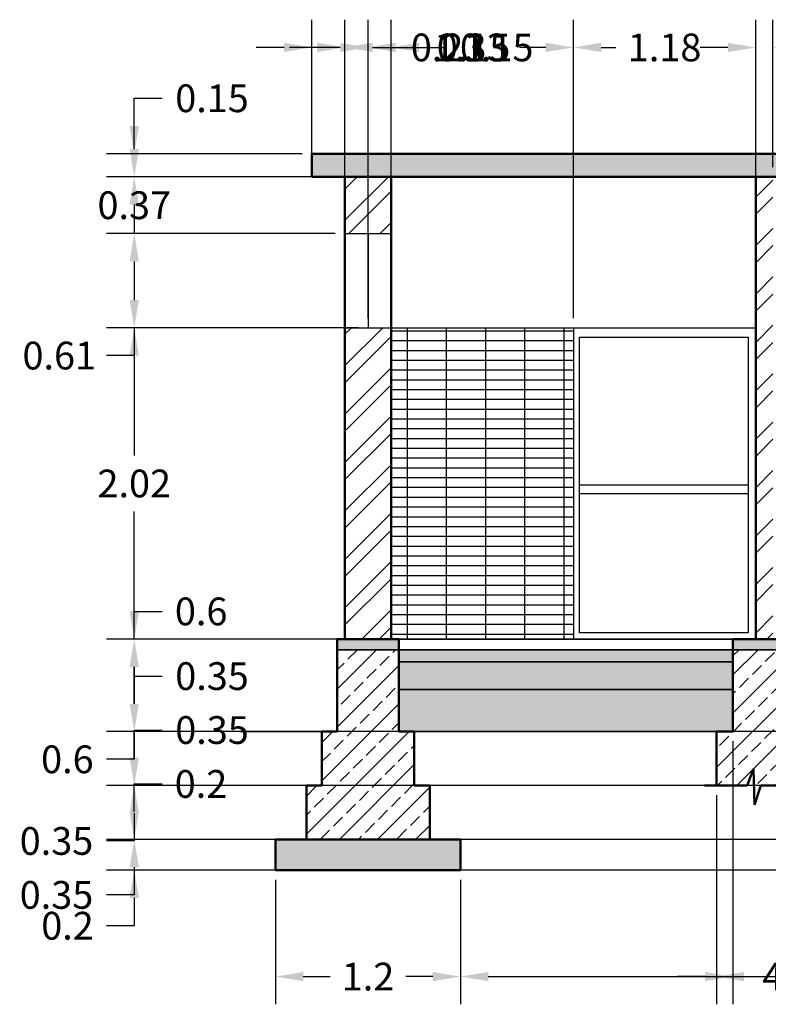
# Model space of a CAD drawing. Units: metres. Extents: x 2294.9 to 2311.3, y 1642.1 to 1648.4.
# Tile 1 of 3: x 2294.9 to 2299.8, y 1642.1 to 1648.4. Entities that reach past the tile are written whole.
import ezdxf

# ---------------------------------------------------------------- set-up
doc = ezdxf.new("R2010")
doc.units = ezdxf.units.M
for name, color, linetype, lineweight in [('A-ANNO-DIMS', 2, 'Continuous', 18), ('A-DOOR', 4, 'Continuous', 25), ('A-FLOR', 3, 'Continuous', 35), ('A-FLOR-PATT', 8, 'Continuous', 13), ('A-GLAZ', 4, 'Continuous', 25), ('A-WALL', 7, 'Continuous', 50), ('A-WALL-PATT', 8, 'Continuous', 13), ('C-TOPO', 8, 'Continuous', 35), ('S-FNDN', 1, 'Continuous', 50), ('S-FNDN-PATT', 8, 'Continuous', 13), ('S-SLAB', 1, 'Continuous', 50), ('S-SLAB-PATT', 8, 'Continuous', 13)]:
    doc.layers.add(name, color=color, linetype=linetype, lineweight=lineweight)
doc.styles.get("Standard").update_dxf_attribs({"font": 'arial.ttf'})
doc.dimstyles.get("Standard").update_dxf_attribs({"dimtxt": 0.18, "dimasz": 0.18, "dimexe": 0.18, "dimexo": 0.0625, "dimgap": 0.09, "dimtad": 0, "dimtih": 1, "dimtoh": 1, "dimdec": 4, "dimzin": 0, "dimdsep": 46, "dimtxsty": 'Standard', "dimcen": 0.09, "dimadec": 0, "dimazin": 0, "dimtfac": 1, "dimtdec": 4, "dimtofl": 0, "dimtmove": 0, "dimatfit": 3, "dimfxl": 1, "dimtolj": 1, "dimtzin": 0, "dimarcsym": 0})

# ---------------------------------------------------------------- blocks, each defined once
blk = doc.blocks.new('FOOTING-PCC-PAD')
for p, q in [((1.1996, 0.1999), (-0.0004, 0.1999)), ((-0.0004, 0.1999), (-0.0004, -0.0001)), ((1.1996, -0.0001), (1.1996, 0.1999)), ((-0.0004, -0.0001), (1.1996, -0.0001))]:
    blk.add_line(p, q)
blk = doc.blocks.new('*D3')
at = {"layer": 'A-ANNO-DIMS', "color": 0, "lineweight": -2, "transparency": 16777216}
for p, q in [((2296.8101, 1647.4894), (2296.8101, 1648.4469)), ((2297.0246, 1647.4894), (2297.0246, 1648.4469)), ((2296.6301, 1648.2669), (2296.4501, 1648.2669)), ((2297.2046, 1648.2669), (2297.3846, 1648.2669))]:
    blk.add_line(p, q, dxfattribs=at)
at = {"layer": 'A-ANNO-DIMS', "color": 0, "transparency": 16777216}
for points in [[(2296.6301, 1648.2969), (2296.6301, 1648.2369), (2296.8101, 1648.2669)], [(2297.2046, 1648.2969), (2297.2046, 1648.2369), (2297.0246, 1648.2669)]]:
    blk.add_solid(points, dxfattribs=at)
at = {"layer": 'Defpoints', "color": 0, "transparency": 16777216}
for p in [(2297.0246, 1648.2669), (2296.8101, 1647.4269), (2297.0246, 1647.4269)]:
    blk.add_point(p, dxfattribs=at)
at = {"layer": 'A-ANNO-DIMS', "color": 0, "transparency": 16777216, "insert": (2297.691, 1648.2669), "char_height": 0.18, "attachment_point": 5}
blk.add_mtext('\\A1;0.21', dxfattribs=at)
blk = doc.blocks.new('*D4')
at = {"layer": 'A-ANNO-DIMS', "color": 0, "lineweight": -2, "transparency": 16777216}
for p, q in [((2297.0246, 1647.1211), (2297.0246, 1648.4469)), ((2297.1746, 1647.1211), (2297.1746, 1648.4469)), ((2296.8446, 1648.2669), (2296.6646, 1648.2669)), ((2297.3546, 1648.2669), (2297.5346, 1648.2669))]:
    blk.add_line(p, q, dxfattribs=at)
at = {"layer": 'A-ANNO-DIMS', "color": 0, "transparency": 16777216}
for points in [[(2296.8446, 1648.2969), (2296.8446, 1648.2369), (2297.0246, 1648.2669)], [(2297.3546, 1648.2969), (2297.3546, 1648.2369), (2297.1746, 1648.2669)]]:
    blk.add_solid(points, dxfattribs=at)
at = {"layer": 'Defpoints', "color": 0, "transparency": 16777216}
for p in [(2297.1746, 1648.2669), (2297.0246, 1647.0586), (2297.1746, 1647.0586)]:
    blk.add_point(p, dxfattribs=at)
at = {"layer": 'A-ANNO-DIMS', "color": 0, "transparency": 16777216, "insert": (2297.8591, 1648.2669), "char_height": 0.18, "attachment_point": 5}
blk.add_mtext('\\A1;0.15', dxfattribs=at)
blk = doc.blocks.new('*D5')
at = {"layer": 'A-ANNO-DIMS', "color": 0, "lineweight": -2, "transparency": 16777216}
for p, q in [((2297.1746, 1647.1211), (2297.1746, 1648.4469)), ((2297.3246, 1647.1211), (2297.3246, 1648.4469)), ((2296.9946, 1648.2669), (2296.8146, 1648.2669)), ((2297.5046, 1648.2669), (2297.6846, 1648.2669))]:
    blk.add_line(p, q, dxfattribs=at)
at = {"layer": 'A-ANNO-DIMS', "color": 0, "transparency": 16777216}
for points in [[(2296.9946, 1648.2969), (2296.9946, 1648.2369), (2297.1746, 1648.2669)], [(2297.5046, 1648.2969), (2297.5046, 1648.2369), (2297.3246, 1648.2669)]]:
    blk.add_solid(points, dxfattribs=at)
at = {"layer": 'Defpoints', "color": 0, "transparency": 16777216}
for p in [(2297.3246, 1648.2669), (2297.1746, 1647.0586), (2297.3246, 1647.0586)]:
    blk.add_point(p, dxfattribs=at)
at = {"layer": 'A-ANNO-DIMS', "color": 0, "transparency": 16777216, "insert": (2298.0091, 1648.2669), "char_height": 0.18, "attachment_point": 5}
blk.add_mtext('\\A1;0.15', dxfattribs=at)
blk = doc.blocks.new('*D6')
at = {"layer": 'A-ANNO-DIMS', "color": 0, "lineweight": -2, "transparency": 16777216}
for p, q in [((2297.1746, 1646.5096), (2297.1746, 1648.4469)), ((2298.5071, 1646.5096), (2298.5071, 1648.4469)), ((2297.3546, 1648.2669), (2297.5255, 1648.2669)), ((2298.3271, 1648.2669), (2298.1561, 1648.2669))]:
    blk.add_line(p, q, dxfattribs=at)
at = {"layer": 'A-ANNO-DIMS', "color": 0, "transparency": 16777216}
for points in [[(2297.3546, 1648.2969), (2297.3546, 1648.2369), (2297.1746, 1648.2669)], [(2298.3271, 1648.2969), (2298.3271, 1648.2369), (2298.5071, 1648.2669)]]:
    blk.add_solid(points, dxfattribs=at)
at = {"layer": 'Defpoints', "color": 0, "transparency": 16777216}
for p in [(2298.5071, 1648.2669), (2297.1746, 1646.4471), (2298.5071, 1646.4471)]:
    blk.add_point(p, dxfattribs=at)
at = {"layer": 'A-ANNO-DIMS', "color": 0, "transparency": 16777216, "insert": (2297.8408, 1648.2669), "char_height": 0.18, "attachment_point": 5}
blk.add_mtext('\\A1;1.33', dxfattribs=at)
blk = doc.blocks.new('*D7')
at = {"layer": 'A-ANNO-DIMS', "color": 0, "lineweight": -2, "transparency": 16777216}
for p, q in [((2298.5071, 1646.5096), (2298.5071, 1648.4469)), ((2299.6895, 1646.5096), (2299.6895, 1648.4469)), ((2298.6871, 1648.2669), (2298.7828, 1648.2669)), ((2299.5095, 1648.2669), (2299.4138, 1648.2669))]:
    blk.add_line(p, q, dxfattribs=at)
at = {"layer": 'A-ANNO-DIMS', "color": 0, "transparency": 16777216}
for points in [[(2298.6871, 1648.2969), (2298.6871, 1648.2369), (2298.5071, 1648.2669)], [(2299.5095, 1648.2969), (2299.5095, 1648.2369), (2299.6895, 1648.2669)]]:
    blk.add_solid(points, dxfattribs=at)
at = {"layer": 'Defpoints', "color": 0, "transparency": 16777216}
for p in [(2299.6895, 1648.2669), (2298.5071, 1646.4471), (2299.6895, 1646.4471)]:
    blk.add_point(p, dxfattribs=at)
at = {"layer": 'A-ANNO-DIMS', "color": 0, "transparency": 16777216, "insert": (2299.0983, 1648.2669), "char_height": 0.18, "attachment_point": 5}
blk.add_mtext('\\A1;1.18', dxfattribs=at)
blk = doc.blocks.new('*D8')
at = {"layer": 'A-ANNO-DIMS', "color": 0, "lineweight": -2, "transparency": 16777216}
for p, q in [((2299.6895, 1647.4894), (2299.6895, 1648.4469)), ((2299.8007, 1647.4894), (2299.8007, 1648.4469)), ((2299.5095, 1648.2669), (2299.3295, 1648.2669)), ((2299.9807, 1648.2669), (2300.1607, 1648.2669))]:
    blk.add_line(p, q, dxfattribs=at)
at = {"layer": 'A-ANNO-DIMS', "color": 0, "transparency": 16777216}
for points in [[(2299.5095, 1648.2969), (2299.5095, 1648.2369), (2299.6895, 1648.2669)], [(2299.9807, 1648.2969), (2299.9807, 1648.2369), (2299.8007, 1648.2669)]]:
    blk.add_solid(points, dxfattribs=at)
at = {"layer": 'Defpoints', "color": 0, "transparency": 16777216}
for p in [(2299.8007, 1648.2669), (2299.6895, 1647.4269), (2299.8007, 1647.4269)]:
    blk.add_point(p, dxfattribs=at)
at = {"layer": 'A-ANNO-DIMS', "color": 0, "transparency": 16777216, "insert": (2300.4671, 1648.2669), "char_height": 0.18, "attachment_point": 5}
blk.add_mtext('\\A1;0.11', dxfattribs=at)
blk = doc.blocks.new('*D18')
at = {"layer": 'A-ANNO-DIMS', "color": 0, "lineweight": -2, "transparency": 16777216}
for p, q in [((2296.5746, 1642.8644), (2296.5746, 1642.0569)), ((2297.7746, 1642.8644), (2297.7746, 1642.0569)), ((2296.7546, 1642.2369), (2296.9301, 1642.2369)), ((2297.5946, 1642.2369), (2297.4191, 1642.2369))]:
    blk.add_line(p, q, dxfattribs=at)
at = {"layer": 'A-ANNO-DIMS', "color": 0, "transparency": 16777216}
for points in [[(2296.7546, 1642.2669), (2296.7546, 1642.2069), (2296.5746, 1642.2369)], [(2297.5946, 1642.2669), (2297.5946, 1642.2069), (2297.7746, 1642.2369)]]:
    blk.add_solid(points, dxfattribs=at)
at = {"layer": 'Defpoints', "color": 0, "transparency": 16777216}
for p in [(2296.5746, 1642.9269), (2297.7746, 1642.9269), (2297.7746, 1642.2369)]:
    blk.add_point(p, dxfattribs=at)
at = {"layer": 'A-ANNO-DIMS', "color": 0, "transparency": 16777216, "insert": (2297.1746, 1642.2369), "char_height": 0.18, "attachment_point": 5}
blk.add_mtext('\\A1;1.2', dxfattribs=at)
blk = doc.blocks.new('*D19')
at = {"layer": 'A-ANNO-DIMS', "color": 0, "lineweight": -2, "transparency": 16777216}
for p, q in [((2297.7746, 1642.8644), (2297.7746, 1642.0569)), ((2302.3014, 1642.8644), (2302.3014, 1642.0569)), ((2297.9546, 1642.2369), (2299.6407, 1642.2369)), ((2302.1214, 1642.2369), (2300.4353, 1642.2369))]:
    blk.add_line(p, q, dxfattribs=at)
at = {"layer": 'A-ANNO-DIMS', "color": 0, "transparency": 16777216}
for points in [[(2297.9546, 1642.2669), (2297.9546, 1642.2069), (2297.7746, 1642.2369)], [(2302.1214, 1642.2669), (2302.1214, 1642.2069), (2302.3014, 1642.2369)]]:
    blk.add_solid(points, dxfattribs=at)
at = {"layer": 'Defpoints', "color": 0, "transparency": 16777216}
for p in [(2297.7746, 1642.9269), (2302.3014, 1642.9269), (2302.3014, 1642.2369)]:
    blk.add_point(p, dxfattribs=at)
at = {"layer": 'A-ANNO-DIMS', "color": 0, "transparency": 16777216, "insert": (2300.038, 1642.2369), "char_height": 0.18, "attachment_point": 5}
blk.add_mtext('\\A1;4.527', dxfattribs=at)
blk = doc.blocks.new('*D23')
at = {"layer": 'A-ANNO-DIMS', "color": 0, "lineweight": -2, "transparency": 16777216}
for p, q in [((2299.5412, 1643.7644), (2299.5412, 1642.0569)), ((2299.9412, 1643.7644), (2299.9412, 1642.0569)), ((2299.3612, 1642.2369), (2299.1812, 1642.2369)), ((2300.1212, 1642.2369), (2300.3012, 1642.2369))]:
    blk.add_line(p, q, dxfattribs=at)
at = {"layer": 'A-ANNO-DIMS', "color": 0, "transparency": 16777216}
for points in [[(2299.3612, 1642.2669), (2299.3612, 1642.2069), (2299.5412, 1642.2369)], [(2300.1212, 1642.2669), (2300.1212, 1642.2069), (2299.9412, 1642.2369)]]:
    blk.add_solid(points, dxfattribs=at)
at = {"layer": 'Defpoints', "color": 0, "transparency": 16777216}
for p in [(2299.5412, 1643.8269), (2299.9412, 1643.8269), (2299.9412, 1642.2369)]:
    blk.add_point(p, dxfattribs=at)
at = {"layer": 'A-ANNO-DIMS', "color": 0, "transparency": 16777216, "insert": (2300.5547, 1642.2369), "char_height": 0.18, "attachment_point": 5}
blk.add_mtext('\\A1;0.4', dxfattribs=at)
blk = doc.blocks.new('*D24')
at = {"layer": 'A-ANNO-DIMS', "color": 0, "lineweight": -2, "transparency": 16777216}
for p, q in [((2299.4343, 1643.4144), (2299.4343, 1642.0569)), ((2300.0343, 1643.4144), (2300.0343, 1642.0569)), ((2299.6143, 1642.2369), (2299.8543, 1642.2369)), ((2300.0343, 1642.2369), (2300.2143, 1642.2369))]:
    blk.add_line(p, q, dxfattribs=at)
at = {"layer": 'A-ANNO-DIMS', "color": 0, "transparency": 16777216}
for points in [[(2299.6143, 1642.2669), (2299.6143, 1642.2069), (2299.4343, 1642.2369)], [(2299.8543, 1642.2669), (2299.8543, 1642.2069), (2300.0343, 1642.2369)]]:
    blk.add_solid(points, dxfattribs=at)
at = {"layer": 'Defpoints', "color": 0, "transparency": 16777216}
for p in [(2299.4343, 1643.4769), (2300.0343, 1643.4769), (2300.0343, 1642.2369)]:
    blk.add_point(p, dxfattribs=at)
at = {"layer": 'A-ANNO-DIMS', "color": 0, "transparency": 16777216, "insert": (2300.4681, 1642.2369), "char_height": 0.18, "attachment_point": 5}
blk.add_mtext('\\A1;0.6', dxfattribs=at)
blk = doc.blocks.new('*D31')
at = {"layer": 'A-ANNO-DIMS', "color": 0, "lineweight": -2, "transparency": 16777216}
for p, q in [((2295.6583, 1644.0069), (2295.6583, 1644.1869)), ((2302.5389, 1643.8269), (2295.4783, 1643.8269)), ((2302.5389, 1643.4769), (2295.4783, 1643.4769)), ((2295.6583, 1643.2969), (2295.6583, 1643.1169)), ((2295.6583, 1643.1169), (2295.4783, 1643.1169))]:
    blk.add_line(p, q, dxfattribs=at)
at = {"layer": 'A-ANNO-DIMS', "color": 0, "transparency": 16777216}
for points in [[(2295.6283, 1644.0069), (2295.6883, 1644.0069), (2295.6583, 1643.8269)], [(2295.6283, 1643.2969), (2295.6883, 1643.2969), (2295.6583, 1643.4769)]]:
    blk.add_solid(points, dxfattribs=at)
at = {"layer": 'Defpoints', "color": 0, "transparency": 16777216}
for p in [(2302.6014, 1643.8269), (2295.6583, 1643.4769), (2302.6014, 1643.4769)]:
    blk.add_point(p, dxfattribs=at)
at = {"layer": 'A-ANNO-DIMS', "color": 0, "transparency": 16777216, "insert": (2295.1539, 1643.1169), "char_height": 0.18, "attachment_point": 5}
blk.add_mtext('\\A1;0.35', dxfattribs=at)
blk = doc.blocks.new('*D32')
at = {"layer": 'A-ANNO-DIMS', "color": 0, "lineweight": -2, "transparency": 16777216}
for p, q in [((2295.6583, 1643.6569), (2295.6583, 1643.8369)), ((2302.4389, 1643.4769), (2295.4783, 1643.4769)), ((2302.4389, 1643.1269), (2295.4783, 1643.1269)), ((2295.6583, 1642.9469), (2295.6583, 1642.7669)), ((2295.6583, 1642.7669), (2295.4783, 1642.7669))]:
    blk.add_line(p, q, dxfattribs=at)
at = {"layer": 'A-ANNO-DIMS', "color": 0, "transparency": 16777216}
for points in [[(2295.6283, 1643.6569), (2295.6883, 1643.6569), (2295.6583, 1643.4769)], [(2295.6283, 1642.9469), (2295.6883, 1642.9469), (2295.6583, 1643.1269)]]:
    blk.add_solid(points, dxfattribs=at)
at = {"layer": 'Defpoints', "color": 0, "transparency": 16777216}
for p in [(2302.5014, 1643.4769), (2295.6583, 1643.1269), (2302.5014, 1643.1269)]:
    blk.add_point(p, dxfattribs=at)
at = {"layer": 'A-ANNO-DIMS', "color": 0, "transparency": 16777216, "insert": (2295.1539, 1642.7669), "char_height": 0.18, "attachment_point": 5}
blk.add_mtext('\\A1;0.35', dxfattribs=at)
blk = doc.blocks.new('*D33')
at = {"layer": 'A-ANNO-DIMS', "color": 0, "lineweight": -2, "transparency": 16777216}
for p, q in [((2295.6583, 1643.3069), (2295.6583, 1643.4869)), ((2302.2389, 1643.1269), (2295.4783, 1643.1269)), ((2302.2389, 1642.9269), (2295.4783, 1642.9269)), ((2295.6583, 1642.7469), (2295.6583, 1642.5669)), ((2295.6583, 1642.5669), (2295.4783, 1642.5669))]:
    blk.add_line(p, q, dxfattribs=at)
at = {"layer": 'A-ANNO-DIMS', "color": 0, "transparency": 16777216}
for points in [[(2295.6283, 1643.3069), (2295.6883, 1643.3069), (2295.6583, 1643.1269)], [(2295.6283, 1642.7469), (2295.6883, 1642.7469), (2295.6583, 1642.9269)]]:
    blk.add_solid(points, dxfattribs=at)
at = {"layer": 'Defpoints', "color": 0, "transparency": 16777216}
for p in [(2302.3014, 1643.1269), (2295.6583, 1642.9269), (2302.3014, 1642.9269)]:
    blk.add_point(p, dxfattribs=at)
at = {"layer": 'A-ANNO-DIMS', "color": 0, "transparency": 16777216, "insert": (2295.2254, 1642.5669), "char_height": 0.18, "attachment_point": 5}
blk.add_mtext('\\A1;0.2', dxfattribs=at)
blk = doc.blocks.new('*D34')
at = {"layer": 'A-ANNO-DIMS', "color": 0, "lineweight": -2, "transparency": 16777216}
for p, q in [((2302.6389, 1644.4269), (2295.4783, 1644.4269)), ((2295.6583, 1644.2469), (2295.6583, 1644.0069)), ((2302.6389, 1643.8269), (2295.4783, 1643.8269)), ((2295.6583, 1643.8269), (2295.6583, 1643.6469)), ((2295.6583, 1643.6469), (2295.4783, 1643.6469))]:
    blk.add_line(p, q, dxfattribs=at)
at = {"layer": 'A-ANNO-DIMS', "color": 0, "transparency": 16777216}
for points in [[(2295.6283, 1644.2469), (2295.6883, 1644.2469), (2295.6583, 1644.4269)], [(2295.6283, 1644.0069), (2295.6883, 1644.0069), (2295.6583, 1643.8269)]]:
    blk.add_solid(points, dxfattribs=at)
at = {"layer": 'Defpoints', "color": 0, "transparency": 16777216}
for p in [(2302.7014, 1644.4269), (2295.6583, 1643.8269), (2302.7014, 1643.8269)]:
    blk.add_point(p, dxfattribs=at)
at = {"layer": 'A-ANNO-DIMS', "color": 0, "transparency": 16777216, "insert": (2295.2245, 1643.6469), "char_height": 0.18, "attachment_point": 5}
blk.add_mtext('\\A1;0.6', dxfattribs=at)
blk = doc.blocks.new('*D44')
at = {"layer": 'A-ANNO-DIMS', "color": 0, "lineweight": -2, "transparency": 16777216}
for p, q in [((2295.6583, 1647.7569), (2295.6583, 1647.9369)), ((2295.6583, 1647.9369), (2295.8383, 1647.9369)), ((2296.7476, 1647.5769), (2295.4783, 1647.5769)), ((2296.7476, 1647.4269), (2295.4783, 1647.4269)), ((2295.6583, 1647.2469), (2295.6583, 1647.0669))]:
    blk.add_line(p, q, dxfattribs=at)
at = {"layer": 'A-ANNO-DIMS', "color": 0, "transparency": 16777216}
for points in [[(2295.6283, 1647.7569), (2295.6883, 1647.7569), (2295.6583, 1647.5769)], [(2295.6283, 1647.2469), (2295.6883, 1647.2469), (2295.6583, 1647.4269)]]:
    blk.add_solid(points, dxfattribs=at)
at = {"layer": 'Defpoints', "color": 0, "transparency": 16777216}
for p in [(2295.6583, 1647.5769), (2296.8101, 1647.5769), (2296.8101, 1647.4269)]:
    blk.add_point(p, dxfattribs=at)
at = {"layer": 'A-ANNO-DIMS', "color": 0, "transparency": 16777216, "insert": (2296.1628, 1647.9369), "char_height": 0.18, "attachment_point": 5}
blk.add_mtext('\\A1;0.15', dxfattribs=at)
blk = doc.blocks.new('*D45')
at = {"layer": 'A-ANNO-DIMS', "color": 0, "lineweight": -2, "transparency": 16777216}
for p, q in [((2295.658308, 1647.606914), (2295.658308, 1647.786914)), ((2296.96211, 1647.426914), (2295.478308, 1647.426914)), ((2296.96211, 1647.058588), (2295.478308, 1647.058588)), ((2295.658308, 1646.878588), (2295.658308, 1646.698588))]:
    blk.add_line(p, q, dxfattribs=at)
at = {"layer": 'A-ANNO-DIMS', "color": 0, "transparency": 16777216}
for points in [[(2295.628308, 1647.606914), (2295.688308, 1647.606914), (2295.658308, 1647.426914)], [(2295.628308, 1646.878588), (2295.688308, 1646.878588), (2295.658308, 1647.058588)]]:
    blk.add_solid(points, dxfattribs=at)
at = {"layer": 'Defpoints', "color": 0, "transparency": 16777216}
for p in [(2297.02461, 1647.426914), (2295.658308, 1647.058588), (2297.02461, 1647.058588)]:
    blk.add_point(p, dxfattribs=at)
at = {"layer": 'A-ANNO-DIMS', "color": 0, "transparency": 16777216, "insert": (2295.658308, 1647.242751), "char_height": 0.18, "attachment_point": 5}
blk.add_mtext('\\A1;0.37', dxfattribs=at)
blk = doc.blocks.new('*D46')
at = {"layer": 'A-ANNO-DIMS', "color": 0, "lineweight": -2, "transparency": 16777216}
for p, q in [((2296.9621, 1647.0586), (2295.4783, 1647.0586)), ((2295.6583, 1646.8786), (2295.6583, 1646.6271)), ((2296.9621, 1646.4471), (2295.4783, 1646.4471)), ((2295.6583, 1646.4471), (2295.6583, 1646.2671)), ((2295.6583, 1646.2671), (2295.4783, 1646.2671))]:
    blk.add_line(p, q, dxfattribs=at)
at = {"layer": 'A-ANNO-DIMS', "color": 0, "transparency": 16777216}
for points in [[(2295.6283, 1646.8786), (2295.6883, 1646.8786), (2295.6583, 1647.0586)], [(2295.6283, 1646.6271), (2295.6883, 1646.6271), (2295.6583, 1646.4471)]]:
    blk.add_solid(points, dxfattribs=at)
at = {"layer": 'Defpoints', "color": 0, "transparency": 16777216}
for p in [(2297.0246, 1647.0586), (2295.6583, 1646.4471), (2297.0246, 1646.4471)]:
    blk.add_point(p, dxfattribs=at)
at = {"layer": 'A-ANNO-DIMS', "color": 0, "transparency": 16777216, "insert": (2295.1719, 1646.2671), "char_height": 0.18, "attachment_point": 5}
blk.add_mtext('\\A1;0.61', dxfattribs=at)
blk = doc.blocks.new('*D47')
at = {"layer": 'A-ANNO-DIMS', "color": 0, "lineweight": -2, "transparency": 16777216}
for p, q in [((2297.1121, 1646.4471), (2295.4783, 1646.4471)), ((2295.6583, 1646.2671), (2295.6583, 1645.6189)), ((2295.6583, 1644.6069), (2295.6583, 1645.2551)), ((2296.9621, 1644.4269), (2295.4783, 1644.4269))]:
    blk.add_line(p, q, dxfattribs=at)
at = {"layer": 'A-ANNO-DIMS', "color": 0, "transparency": 16777216}
for points in [[(2295.6283, 1646.2671), (2295.6883, 1646.2671), (2295.6583, 1646.4471)], [(2295.6283, 1644.6069), (2295.6883, 1644.6069), (2295.6583, 1644.4269)]]:
    blk.add_solid(points, dxfattribs=at)
at = {"layer": 'Defpoints', "color": 0, "transparency": 16777216}
for p in [(2295.6583, 1646.4471), (2297.1746, 1646.4471), (2297.0246, 1644.4269)]:
    blk.add_point(p, dxfattribs=at)
at = {"layer": 'A-ANNO-DIMS', "color": 0, "transparency": 16777216, "insert": (2295.6583, 1645.437), "char_height": 0.18, "attachment_point": 5}
blk.add_mtext('\\A1;2.02', dxfattribs=at)
blk = doc.blocks.new('*D48')
at = {"layer": 'A-ANNO-DIMS', "color": 0, "lineweight": -2, "transparency": 16777216}
for p, q in [((2295.6583, 1644.4269), (2295.6583, 1644.6069)), ((2295.6583, 1644.6069), (2295.8383, 1644.6069)), ((2296.9121, 1644.4269), (2295.4783, 1644.4269)), ((2295.6583, 1644.0069), (2295.6583, 1644.2469)), ((2296.2858, 1643.8269), (2295.4783, 1643.8269))]:
    blk.add_line(p, q, dxfattribs=at)
at = {"layer": 'A-ANNO-DIMS', "color": 0, "transparency": 16777216}
for points in [[(2295.6283, 1644.2469), (2295.6883, 1644.2469), (2295.6583, 1644.4269)], [(2295.6283, 1644.0069), (2295.6883, 1644.0069), (2295.6583, 1643.8269)]]:
    blk.add_solid(points, dxfattribs=at)
at = {"layer": 'Defpoints', "color": 0, "transparency": 16777216}
for p in [(2295.6583, 1644.4269), (2296.9746, 1644.4269), (2296.3483, 1643.8269)]:
    blk.add_point(p, dxfattribs=at)
at = {"layer": 'A-ANNO-DIMS', "color": 0, "transparency": 16777216, "insert": (2296.0921, 1644.6069), "char_height": 0.18, "attachment_point": 5}
blk.add_mtext('\\A1;0.6', dxfattribs=at)
blk = doc.blocks.new('*D49')
at = {"layer": 'A-ANNO-DIMS', "color": 0, "lineweight": -2, "transparency": 16777216}
for p, q in [((2295.6583, 1644.0069), (2295.6583, 1644.1869)), ((2295.6583, 1644.1869), (2295.8383, 1644.1869)), ((2296.2858, 1643.8269), (2295.4783, 1643.8269)), ((2296.7121, 1643.4769), (2295.4783, 1643.4769)), ((2295.6583, 1643.2969), (2295.6583, 1643.1169))]:
    blk.add_line(p, q, dxfattribs=at)
at = {"layer": 'A-ANNO-DIMS', "color": 0, "transparency": 16777216}
for points in [[(2295.6283, 1644.0069), (2295.6883, 1644.0069), (2295.6583, 1643.8269)], [(2295.6283, 1643.2969), (2295.6883, 1643.2969), (2295.6583, 1643.4769)]]:
    blk.add_solid(points, dxfattribs=at)
at = {"layer": 'Defpoints', "color": 0, "transparency": 16777216}
for p in [(2295.6583, 1643.8269), (2296.3483, 1643.8269), (2296.7746, 1643.4769)]:
    blk.add_point(p, dxfattribs=at)
at = {"layer": 'A-ANNO-DIMS', "color": 0, "transparency": 16777216, "insert": (2296.1628, 1644.1869), "char_height": 0.18, "attachment_point": 5}
blk.add_mtext('\\A1;0.35', dxfattribs=at)
blk = doc.blocks.new('*D50')
at = {"layer": 'A-ANNO-DIMS', "color": 0, "lineweight": -2, "transparency": 16777216}
for p, q in [((2295.6583, 1643.6569), (2295.6583, 1643.8369)), ((2295.6583, 1643.8369), (2295.8383, 1643.8369)), ((2296.7121, 1643.4769), (2295.4783, 1643.4769)), ((2296.5121, 1643.1269), (2295.4783, 1643.1269)), ((2295.6583, 1642.9469), (2295.6583, 1642.7669))]:
    blk.add_line(p, q, dxfattribs=at)
at = {"layer": 'A-ANNO-DIMS', "color": 0, "transparency": 16777216}
for points in [[(2295.6283, 1643.6569), (2295.6883, 1643.6569), (2295.6583, 1643.4769)], [(2295.6283, 1642.9469), (2295.6883, 1642.9469), (2295.6583, 1643.1269)]]:
    blk.add_solid(points, dxfattribs=at)
at = {"layer": 'Defpoints', "color": 0, "transparency": 16777216}
for p in [(2295.6583, 1643.4769), (2296.7746, 1643.4769), (2296.5746, 1643.1269)]:
    blk.add_point(p, dxfattribs=at)
at = {"layer": 'A-ANNO-DIMS', "color": 0, "transparency": 16777216, "insert": (2296.1628, 1643.8369), "char_height": 0.18, "attachment_point": 5}
blk.add_mtext('\\A1;0.35', dxfattribs=at)
blk = doc.blocks.new('*D51')
at = {"layer": 'A-ANNO-DIMS', "color": 0, "lineweight": -2, "transparency": 16777216}
for p, q in [((2295.6583, 1643.3069), (2295.6583, 1643.4869)), ((2295.6583, 1643.4869), (2295.8383, 1643.4869)), ((2296.5121, 1643.1269), (2295.4783, 1643.1269)), ((2296.5121, 1642.9269), (2295.4783, 1642.9269)), ((2295.6583, 1642.7469), (2295.6583, 1642.5669))]:
    blk.add_line(p, q, dxfattribs=at)
at = {"layer": 'A-ANNO-DIMS', "color": 0, "transparency": 16777216}
for points in [[(2295.6283, 1643.3069), (2295.6883, 1643.3069), (2295.6583, 1643.1269)], [(2295.6283, 1642.7469), (2295.6883, 1642.7469), (2295.6583, 1642.9269)]]:
    blk.add_solid(points, dxfattribs=at)
at = {"layer": 'Defpoints', "color": 0, "transparency": 16777216}
for p in [(2295.6583, 1643.1269), (2296.5746, 1643.1269), (2296.5746, 1642.9269)]:
    blk.add_point(p, dxfattribs=at)
at = {"layer": 'A-ANNO-DIMS', "color": 0, "transparency": 16777216, "insert": (2296.0912, 1643.4869), "char_height": 0.18, "attachment_point": 5}
blk.add_mtext('\\A1;0.2', dxfattribs=at)

msp = doc.modelspace()

# ---------------------------------------------------------------- hatches: boundary and pattern name
at = {"layer": 'A-FLOR-PATT'}
h = msp.add_hatch(dxfattribs=at)
h.set_pattern_fill('JIS_STN_2.5', color=256, scale=0.07)
h.paths.add_polyline_path([(2297.3746, 1644.3583), (2296.9746, 1644.3583), (2296.9746, 1644.3269), (2296.9746, 1643.8269), (2296.8746, 1643.8269), (2296.8746, 1643.4769), (2296.7746, 1643.4769), (2296.7746, 1643.1269), (2297.5746, 1643.1269), (2297.5746, 1643.4769), (2297.4746, 1643.4769), (2297.4746, 1643.8269), (2297.3746, 1643.8269)])
h.paths.add_polyline_path([(2300.0343, 1643.8269), (2299.9412, 1643.8269), (2299.9412, 1644.3583), (2299.5412, 1644.3583), (2299.5412, 1643.8269), (2299.4343, 1643.8269), (2299.4343, 1643.4769), (2299.6329, 1643.4769), (2299.6744, 1643.5859), (2299.6809, 1643.3504), (2299.7223, 1643.4769), (2300.0343, 1643.4769)])
h.paths.add_polyline_path([(2303.2014, 1643.8269), (2303.1014, 1643.8269), (2303.1014, 1644.3583), (2302.7014, 1644.3583), (2302.7014, 1643.8269), (2302.6014, 1643.8269), (2302.6014, 1643.4769), (2302.5014, 1643.4769), (2302.5014, 1643.1269), (2303.3014, 1643.1269), (2303.3014, 1643.4769), (2303.2014, 1643.4769)])
h.paths.add_polyline_path([(2308.9253, 1643.8269), (2308.8253, 1643.8269), (2308.8253, 1644.3583), (2308.4253, 1644.3583), (2308.4253, 1643.8269), (2308.3253, 1643.8269), (2308.3253, 1643.4769), (2308.2253, 1643.4769), (2308.2253, 1643.1269), (2309.0253, 1643.1269), (2309.0253, 1643.4769), (2308.9253, 1643.4769)])
h = msp.add_hatch(dxfattribs=at)
h.set_pattern_fill('AR-SAND', color=256, scale=0.001)
h.paths.add_polyline_path([(2299.5412, 1644.3583), (2297.3746, 1644.3583), (2297.3746, 1644.2797), (2299.5412, 1644.2797)])
h = msp.add_hatch(dxfattribs=at)
h.set_pattern_fill('AR-CONC', color=256, scale=0.002)
h.paths.add_polyline_path([(2299.5412, 1644.2797), (2297.3746, 1644.2797), (2297.3746, 1644.1004), (2299.5412, 1644.1004)])
h.paths.add_polyline_path([(2302.7014, 1644.2797), (2299.9412, 1644.2797), (2299.9412, 1644.1004), (2302.7014, 1644.1004)])
h.paths.add_polyline_path([(2308.4253, 1644.2797), (2303.1014, 1644.2797), (2303.1014, 1644.1004), (2308.4253, 1644.1004)])
h = msp.add_hatch(dxfattribs=at)
h.set_pattern_fill('GRAVEL', color=256, scale=0.01)
h.set_pattern_definition([(228.0127875, (0.18288, 0.254), (-2.03200000016, -2.28599999986), [0.034172144, -3.383048364]), (184.969741, (0.16002, 0.2286), (3.047999998794, 0.25400001447), [0.058640472, -5.80540489]), (132.5104471, (0.1016, 0.22352), (2.54000000107, -2.793999999025), [0.041348152, -4.09347228]), (267.273689, (0.00254, 0.16002), (0.25400000053, 5.079999999973), [0.053400452, -5.286643743]), (292.8336542, (0, 0.10668), (-1.270000000106, 3.047999999956), [0.05236337, -5.183980775]), (357.273689, (0.02032, 0.05842), (-5.079999999973, 0.25400000053), [0.053400452, -5.286643743]), (37.69424047, (0.07366, 0.05588), (-3.301999999854, -2.54000000019), [0.070619366, -6.991311531]), (72.25532837, (0.12954, 0.09906), (1.778000000478, 5.587999999848), [0.066671952, -6.60052566]), (121.4295656, (0.14986, 0.16256), (-2.03200000029, 3.301999999823), [0.0535813, -5.30455457]), (175.2363583, (0.12192, 0.20828), (2.79399999996, -0.25400000044), [0.061171328, -2.997393695]), (222.3974378, (0.06096, 0.21336), (-3.047999999902, -2.794000000106), [0.079107792, -7.831677251]), (138.8140748, (0.254, 0.15748), (-1.7779999999, 1.52400000012), [0.027000454, -2.673056582]), (171.4692344, (0.23368, 0.17526), (3.30200000009, -0.507999999424), [0.051368198, -5.0854639]), (225, (0.18288, 0.18288), (0, -0.254), [0.035920934, -0.32328931]), (203.1985905, (0.1651, 0.21336), (1.27000000003, 0.5079999999), [0.019344132, -1.915062237]), (291.8014095, (0.14732, 0.20574), (-0.25400000005, 0.762), [0.027356562, -1.3404753]), (30.9637565, (0.15748, 0.18034), (0.762, 0.508), [0.044431966, -1.436629815]), (161.5650512, (0.19558, 0.2032), (0.508, -0.254), [0.032128714, -0.771089812]), (16.38954033, (0, 0.20574), (2.54, 0.762), [0.0450088, -4.455882667]), (70.34617594, (0.04318, 0.21844), (-1.01600000009, -2.79399999997), [0.037759894, -3.738221568]), (293.1985905, (0.19558, 0.254), (-0.5079999999, 1.27000000004), [0.03868801, -1.89571836]), (343.61045967, (0.21082, 0.21844), (-2.54000000005, 0.76199999982), [0.0450088, -4.455882667]), (339.4439548, (0, 0.04826), (-1.27, 0.508), [0.04340352, -2.126773431]), (294.7751406, (0.04064, 0.03302), (-1.27000000151, 2.79399999931), [0.036367212, -3.600359338]), (66.8014095, (0.19812, 0), (0.50799999992, 1.27000000003), [0.03868801, -1.89571836]), (17.35402464, (0.21336, 0.03556), (-3.301999999934, -1.01600000021), [0.042578274, -4.215237598]), (69.4439548, (0.07366, 0), (-0.508, -1.27), [0.02170176, -2.148475191]), (101.3099325, (0.18288, 0), (-0.254, 1.016), [0.01295146, -1.282199496]), (165.9637565, (0.18034, 0.0127), (0.762, -0.254), [0.05236337, -0.99490546]), (186.00900596, (0.12954, 0.0254), (2.539999999987, 0.25400000013), [0.0485267, -4.804136486]), (303.6900675, (0.15748, 0.15748), (-0.254, 0.508), [0.036632388, -0.879177636]), (353.1572266, (0.1778, 0.127), (4.318000000027, -0.507999999774), [0.063955676, -6.331600907]), (60.9453959, (0.2413, 0.11938), (-1.01600000003, -1.77799999998), [0.026150824, -2.588939232]), (90, (0.254, 0.14224), (-0.254, 0.254), [0.01524, -0.23876]), (120.25643716, (0.12446, 0.03302), (1.01599999988, -1.77800000007), [0.035286696, -3.493394077]), (48.0127875, (0.10668, 0.0635), (2.03200000017, 2.28599999985), [0.068344288, -3.34887622]), (0, (0.1524, 0.1143), (0.254, 0.254), [0.06604, -0.18796]), (325.3048465, (0.21844, 0.1143), (2.54000000096, -1.77799999863), [0.040160956, -3.975931672]), (254.0546041, (0.25146, 0.09144), (-0.254, -1.016), [0.036982908, -1.812165004]), (207.64597536, (0.2413, 0.05588), (-4.826000000177, -2.539999999663), [0.06021451, -5.961246442]), (175.42607874, (0.18796, 0.02794), (-3.302, 0.254), [0.063702946, -6.306584646])])
h.paths.add_polyline_path([(2299.5412, 1644.1004), (2297.3746, 1644.1004), (2297.3746, 1643.8269), (2297.4746, 1643.8269), (2299.5412, 1643.8269)])
h.paths.add_polyline_path([(2302.7014, 1644.1004), (2299.9412, 1644.1004), (2299.9412, 1643.8269), (2302.7014, 1643.8269)])
h.paths.add_polyline_path([(2308.4253, 1644.1004), (2303.1014, 1644.1004), (2303.1014, 1643.8269), (2308.4253, 1643.8269)])
at = {"layer": 'A-GLAZ'}
h = msp.add_hatch(dxfattribs=at)
h.set_pattern_fill('GRATE', color=256, scale=0.08)
h.paths.add_polyline_path([(2298.5071, 1646.4471), (2297.3246, 1646.4471), (2297.3246, 1644.4269), (2297.3746, 1644.4269), (2298.5071, 1644.4269)])
at = {"layer": 'A-WALL-PATT'}
h = msp.add_hatch(dxfattribs=at)
h.set_pattern_fill('STEEL', color=256, scale=0.07)
h.set_pattern_definition([(45, (0, 0), (-0.157154482, 0.157154482), []), (45, (0, 0.11113), (-0.157154482, 0.157154482), [])])
h.paths.add_polyline_path([(2297.3246, 1646.4471), (2297.0246, 1646.4471), (2297.0246, 1644.4269), (2297.3246, 1644.4269)])
h.paths.add_polyline_path([(2297.3246, 1647.4269), (2297.1746, 1647.4269), (2297.0246, 1647.4269), (2297.0246, 1647.0586), (2297.3246, 1647.0586)])
h.paths.add_polyline_path([(2299.8007, 1647.4269), (2299.6895, 1647.4269), (2299.6895, 1644.4269), (2299.7412, 1644.4269), (2299.8007, 1644.4269)])
h.paths.add_polyline_path([(2303.0514, 1646.4441), (2303.0514, 1647.4269), (2302.7514, 1647.4269), (2302.7514, 1644.4269), (2303.0514, 1644.4269)])
at = {"layer": 'S-FNDN-PATT'}
h = msp.add_hatch(dxfattribs=at)
h.set_pattern_fill('AR-CONC', color=256, scale=0.001)
h.paths.add_polyline_path([(2297.7746, 1643.1269), (2296.5746, 1643.1269), (2296.5746, 1642.9269), (2297.7746, 1642.9269)])
h.paths.add_polyline_path([(2303.5014, 1643.1269), (2302.3014, 1643.1269), (2302.3014, 1642.9269), (2303.5014, 1642.9269)])
h.paths.add_polyline_path([(2309.2253, 1643.1269), (2308.0253, 1643.1269), (2308.0253, 1642.9269), (2309.2253, 1642.9269)])
h.paths.add_polyline_path([(2297.3746, 1644.4269), (2297.3246, 1644.4269), (2297.0246, 1644.4269), (2296.9746, 1644.4269), (2296.9746, 1644.3583), (2297.3746, 1644.3583)])
h.paths.add_polyline_path([(2299.9412, 1644.4269), (2299.7412, 1644.4269), (2299.5412, 1644.4269), (2299.5412, 1644.3583), (2299.9412, 1644.3583)])
h.paths.add_polyline_path([(2303.1014, 1644.4269), (2303.0514, 1644.4269), (2302.7514, 1644.4269), (2302.7014, 1644.4269), (2302.7014, 1644.3583), (2303.1014, 1644.3583)])
h.paths.add_polyline_path([(2308.8253, 1644.4269), (2308.7753, 1644.4269), (2308.4753, 1644.4269), (2308.4253, 1644.4269), (2308.4253, 1644.3583), (2308.8253, 1644.3583)])
at = {"layer": 'S-SLAB-PATT'}
h = msp.add_hatch(dxfattribs=at)
h.set_pattern_fill('AR-CONC', color=256, scale=0.002)
h.paths.add_polyline_path([(2309.2101, 1647.5769), (2296.8101, 1647.5769), (2296.8101, 1647.4269), (2297.1746, 1647.4269), (2308.6282, 1647.4269), (2309.2101, 1647.4269)])

# ---------------------------------------------------------------- linework, layer by layer
at = {"layer": 'A-DOOR'}
for p, q in [((2298.5462, 1645.4275), (2299.6413, 1645.4275)), ((2298.5462, 1645.3715), (2299.6413, 1645.3715))]:
    msp.add_line(p, q, dxfattribs=at)
msp.add_lwpolyline([(2298.5462, 1646.3871), (2299.6413, 1646.3871), (2299.6413, 1644.4679), (2298.5462, 1644.4679)], close=True, dxfattribs=at)
at = {"layer": 'A-FLOR'}
for p, q in [((2296.9746, 1644.4269), (2296.9746, 1644.3269)), ((2297.3746, 1644.4269), (2302.7514, 1644.4269)), ((2296.9746, 1644.3583), (2308.8253, 1644.3583)), ((2297.3746, 1644.2797), (2299.5412, 1644.2797)), ((2297.3746, 1644.1004), (2299.5412, 1644.1004)), ((2297.4746, 1643.8269), (2299.5412, 1643.8269))]:
    msp.add_line(p, q, dxfattribs=at)
at = {"layer": 'A-GLAZ'}
for p, q in [((2297.0246, 1647.0586), (2297.3246, 1647.0586)), ((2297.1746, 1647.0586), (2297.1746, 1646.4471)), ((2297.0246, 1646.4471), (2299.6895, 1646.4471)), ((2298.5071, 1646.4471), (2298.5071, 1644.4269))]:
    msp.add_line(p, q, dxfattribs=at)
at = {"layer": 'A-WALL'}
for p, q in [((2297.0246, 1644.4269), (2297.0246, 1647.4269)), ((2297.3246, 1647.4269), (2297.0246, 1647.4269)), ((2297.3246, 1644.4269), (2297.3246, 1647.4269)), ((2299.6895, 1647.4269), (2299.6895, 1644.4269)), ((2297.0246, 1644.4269), (2297.3246, 1644.4269)), ((2299.7412, 1644.4269), (2299.6697, 1644.4269))]:
    msp.add_line(p, q, dxfattribs=at)
at = {"layer": 'C-TOPO'}
msp.add_line((2296.8746, 1643.8269), (2296.3483, 1643.8269), dxfattribs=at)
at = {"layer": 'S-FNDN'}
for p, q in [((2296.9746, 1643.8269), (2296.9746, 1644.4269)), ((2296.9746, 1644.4269), (2297.0246, 1644.4269)), ((2297.3246, 1644.4269), (2297.3746, 1644.4269)), ((2297.3746, 1644.4269), (2297.3746, 1643.8269)), ((2299.7412, 1644.4269), (2299.5412, 1644.4269)), ((2299.5412, 1644.4269), (2299.5412, 1643.8269)), ((2299.7412, 1644.4269), (2299.9412, 1644.4269)), ((2296.8746, 1643.4769), (2296.8746, 1643.8269)), ((2296.8746, 1643.8269), (2296.9746, 1643.8269)), ((2297.3746, 1643.8269), (2297.4746, 1643.8269)), ((2297.4746, 1643.8269), (2297.4746, 1643.4769)), ((2299.5412, 1643.8269), (2299.4343, 1643.8269)), ((2299.4343, 1643.8269), (2299.4343, 1643.4769)), ((2299.6329, 1643.4769), (2299.6744, 1643.5859)), ((2299.6744, 1643.5859), (2299.6809, 1643.3504)), ((2296.7746, 1643.1269), (2296.7746, 1643.4769)), ((2296.7746, 1643.4769), (2296.8746, 1643.4769)), ((2297.4746, 1643.4769), (2297.5746, 1643.4769)), ((2297.5746, 1643.4769), (2297.5746, 1643.1269)), ((2299.3561, 1643.4769), (2299.6329, 1643.4769)), ((2299.6809, 1643.3504), (2299.7223, 1643.4769)), ((2299.7223, 1643.4769), (2300.1401, 1643.4769))]:
    msp.add_line(p, q, dxfattribs=at)
at = {"layer": 'S-SLAB'}
for p, q in [((2296.8101, 1647.4269), (2296.8101, 1647.5769)), ((2296.8101, 1647.5769), (2309.2101, 1647.5769)), ((2297.1746, 1647.4269), (2296.8101, 1647.4269)), ((2297.1746, 1647.4269), (2308.6282, 1647.4269)), ((2309.2101, 1647.4269), (2297.3246, 1647.4269))]:
    msp.add_line(p, q, dxfattribs=at)

# ---------------------------------------------------------------- block references
at = {"layer": 'S-FNDN'}
msp.add_blockref('FOOTING-PCC-PAD', (2296.575, 1642.927), dxfattribs=at)

# ---------------------------------------------------------------- dimensions: what is measured, and where the dimension line sits
at = {"layer": 'A-ANNO-DIMS'}
for base, p1, p2, override, picture, middle in [((2297.0246, 1648.2669), (2296.8101, 1647.4269), (2297.0246, 1647.4269), {"dimdec": 2, "dimlfac": 1, "dimrnd": 0, "dimzin": 0, "dimdsep": 46, "dimlunit": 2}, '*D3', (2297.691, 1648.2669)), ((2297.1746, 1648.2669), (2297.0246, 1647.0586), (2297.1746, 1647.0586), {"dimdec": 2, "dimlfac": 1, "dimrnd": 0, "dimzin": 0, "dimdsep": 46, "dimlunit": 2}, '*D4', (2297.8591, 1648.2669)), ((2297.3246, 1648.2669), (2297.1746, 1647.0586), (2297.3246, 1647.0586), {"dimdec": 2, "dimlfac": 1, "dimrnd": 0, "dimzin": 0, "dimdsep": 46, "dimlunit": 2}, '*D5', (2298.0091, 1648.2669)), ((2298.5071, 1648.2669), (2297.1746, 1646.4471), (2298.5071, 1646.4471), {"dimdec": 2, "dimlfac": 1, "dimrnd": 0, "dimzin": 0, "dimdsep": 46, "dimlunit": 2}, '*D6', (2297.8408, 1648.2669)), ((2299.6895, 1648.2669), (2298.5071, 1646.4471), (2299.6895, 1646.4471), {"dimdec": 2, "dimlfac": 1, "dimrnd": 0, "dimzin": 0, "dimdsep": 46, "dimlunit": 2}, '*D7', (2299.0983, 1648.2669)), ((2299.8007, 1648.2669), (2299.6895, 1647.4269), (2299.8007, 1647.4269), {"dimdec": 2, "dimlfac": 1, "dimrnd": 0, "dimzin": 0, "dimdsep": 46, "dimlunit": 2}, '*D8', (2300.4671, 1648.2669)), ((2299.9412, 1642.2369), (2299.5412, 1643.8269), (2299.9412, 1643.8269), {"dimdec": 1, "dimlfac": 1, "dimrnd": 0, "dimzin": 0, "dimdsep": 46, "dimlunit": 2}, '*D23', (2300.5547, 1642.2369)), ((2300.0343, 1642.2369), (2299.4343, 1643.4769), (2300.0343, 1643.4769), {"dimdec": 1, "dimlfac": 1, "dimrnd": 0, "dimzin": 0, "dimdsep": 46, "dimlunit": 2}, '*D24', (2300.4681, 1642.2369)), ((2297.7746, 1642.2369), (2296.5746, 1642.9269), (2297.7746, 1642.9269), {"dimdec": 1, "dimlfac": 1, "dimrnd": 0, "dimzin": 0, "dimdsep": 46, "dimlunit": 2}, '*D18', (2297.1746, 1642.2369)), ((2302.3014, 1642.2369), (2297.7746, 1642.9269), (2302.3014, 1642.9269), {"dimdec": 3, "dimlfac": 1, "dimrnd": 0, "dimzin": 0, "dimdsep": 46, "dimlunit": 2}, '*D19', (2300.038, 1642.2369))]:
    dim = msp.add_linear_dim(base=base, p1=p1, p2=p2, dimstyle='Standard', override=override, dxfattribs=at)
    dim.commit()
    dim.dimension.update_dxf_attribs({"geometry": picture, "text_midpoint": middle})
for base, p1, p2, override, picture, middle in [((2295.6583, 1647.5769), (2296.8101, 1647.4269), (2296.8101, 1647.5769), {"dimdec": 2, "dimlfac": 1, "dimrnd": 0, "dimzin": 0, "dimdsep": 46, "dimlunit": 2}, '*D44', (2296.1628, 1647.9369)), ((2295.6583, 1647.0586), (2297.0246, 1647.4269), (2297.0246, 1647.0586), {"dimdec": 2, "dimlfac": 1, "dimrnd": 0, "dimzin": 0, "dimdsep": 46, "dimlunit": 2}, '*D45', (2295.6583, 1647.2428)), ((2295.6583, 1646.4471), (2297.0246, 1647.0586), (2297.0246, 1646.4471), {"dimdec": 2, "dimlfac": 1, "dimrnd": 0, "dimzin": 0, "dimdsep": 46, "dimlunit": 2}, '*D46', (2295.1719, 1646.2671)), ((2295.6583, 1646.4471), (2297.0246, 1644.4269), (2297.1746, 1646.4471), {"dimdec": 2, "dimlfac": 1, "dimrnd": 0, "dimzin": 0, "dimdsep": 46, "dimlunit": 2}, '*D47', (2295.6583, 1645.437)), ((2295.6583, 1644.4269), (2296.3483, 1643.8269), (2296.9746, 1644.4269), {"dimdec": 1, "dimlfac": 1, "dimrnd": 0, "dimzin": 0, "dimdsep": 46, "dimlunit": 2}, '*D48', (2296.0921, 1644.6069)), ((2295.6583, 1643.8269), (2302.7014, 1644.4269), (2302.7014, 1643.8269), {"dimdec": 1, "dimlfac": 1, "dimrnd": 0, "dimzin": 0, "dimdsep": 46, "dimlunit": 2}, '*D34', (2295.2245, 1643.6469)), ((2295.6583, 1643.8269), (2296.7746, 1643.4769), (2296.3483, 1643.8269), {"dimdec": 2, "dimlfac": 1, "dimrnd": 0, "dimzin": 0, "dimdsep": 46, "dimlunit": 2}, '*D49', (2296.1628, 1644.1869)), ((2295.6583, 1643.4769), (2302.6014, 1643.8269), (2302.6014, 1643.4769), {"dimdec": 2, "dimlfac": 1, "dimrnd": 0, "dimzin": 0, "dimdsep": 46, "dimlunit": 2}, '*D31', (2295.1539, 1643.1169)), ((2295.6583, 1643.4769), (2296.5746, 1643.1269), (2296.7746, 1643.4769), {"dimdec": 2, "dimlfac": 1, "dimrnd": 0, "dimzin": 0, "dimdsep": 46, "dimlunit": 2}, '*D50', (2296.1628, 1643.8369)), ((2295.6583, 1643.1269), (2302.5014, 1643.4769), (2302.5014, 1643.1269), {"dimdec": 2, "dimlfac": 1, "dimrnd": 0, "dimzin": 0, "dimdsep": 46, "dimlunit": 2}, '*D32', (2295.1539, 1642.7669)), ((2295.6583, 1643.1269), (2296.5746, 1642.9269), (2296.5746, 1643.1269), {"dimdec": 1, "dimlfac": 1, "dimrnd": 0, "dimzin": 0, "dimdsep": 46, "dimlunit": 2}, '*D51', (2296.0912, 1643.4869)), ((2295.6583, 1642.9269), (2302.3014, 1643.1269), (2302.3014, 1642.9269), {"dimdec": 1, "dimlfac": 1, "dimrnd": 0, "dimzin": 0, "dimdsep": 46, "dimlunit": 2}, '*D33', (2295.2254, 1642.5669))]:
    dim = msp.add_linear_dim(base=base, p1=p1, p2=p2, angle=90, dimstyle='Standard', override=override, dxfattribs=at)
    dim.commit()
    dim.dimension.update_dxf_attribs({"geometry": picture, "text_midpoint": middle})

doc.saveas('drawing.dxf')
